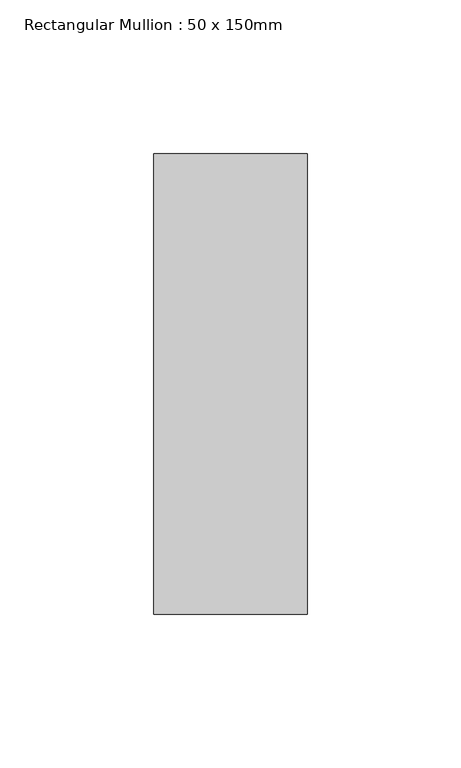
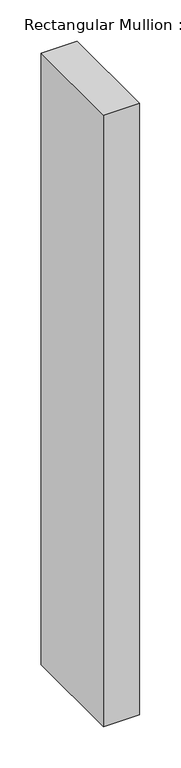
"""IFC4 building model written with IfcOpenShell, lengths in millimetres: member geometry, Rectangular Mullion : 50 x 150mm."""

from ifc_helpers import new_model, si_unit, frame, origin, place, context, project, spatial, polyline, outline, extrude, source, transform, mapped, element, save


def rectangular_mullion_50_x_150mm_3ddb3363(model_context):
    return source(origin(), model_context, "Body", "SweptSolid", [
        extrude(outline(polyline([(25.0, 75.0), (25.0, -75.0), (-25.0, -75.0), (-25.0, 75.0), (25.0, 75.0)])), frame((0.0, 0.0, -900.0), z_axis=(0.0, 0.0, 1.0), x_axis=(1.0, 0.0, 0.0)), (0.0, 0.0, 1.0), 900.0),
    ])


if __name__ == "__main__":
    model = new_model("IFC4")
    model_context = context("Model", 3, world=origin())
    ifc_project = project(units=[si_unit("LENGTHUNIT", "METRE", prefix="MILLI")], contexts=[model_context])
    site = spatial("IfcSite", under=ifc_project)
    building = spatial("IfcBuilding", under=site)
    placement = place(None, origin())
    rectangular_mullion_50_x_150mm_shape = rectangular_mullion_50_x_150mm_3ddb3363(model_context)
    element("IfcMember", 1, ObjectType="Rectangular Mullion : 50 x 150mm", at=placement, inside=building, context=model_context, shape_type="MappedRepresentation", body=[
        mapped(rectangular_mullion_50_x_150mm_shape, transform((0.0, 0.0, 0.0), x_axis=(1.0, 0.0, 0.0), y_axis=(0.0, 1.0, 0.0), z_axis=(0.0, 0.0, 1.0))),
    ])
    save(model, "model.ifc")

# Revit data of these elements
# Type "Rectangular Mullion : 50 x 150mm"
#   built-in parameter 1007304 = 0.492126 (stored number, unit not read)
#   built-in parameter 1007301 = 0.082021 (stored number, unit not read)
#   built-in parameter 1007300 = 0.082021 (stored number, unit not read)
# Element 1 (IfcMember, "Rectangular Mullion : 50 x 150mm")
#   Materials on its faces: "Aluminium"
# Materials
#   "Aluminium": class "Metal", colour RGB 247 247 247, transparency 0, Description = "Aluminium 6061", Cost = 0
